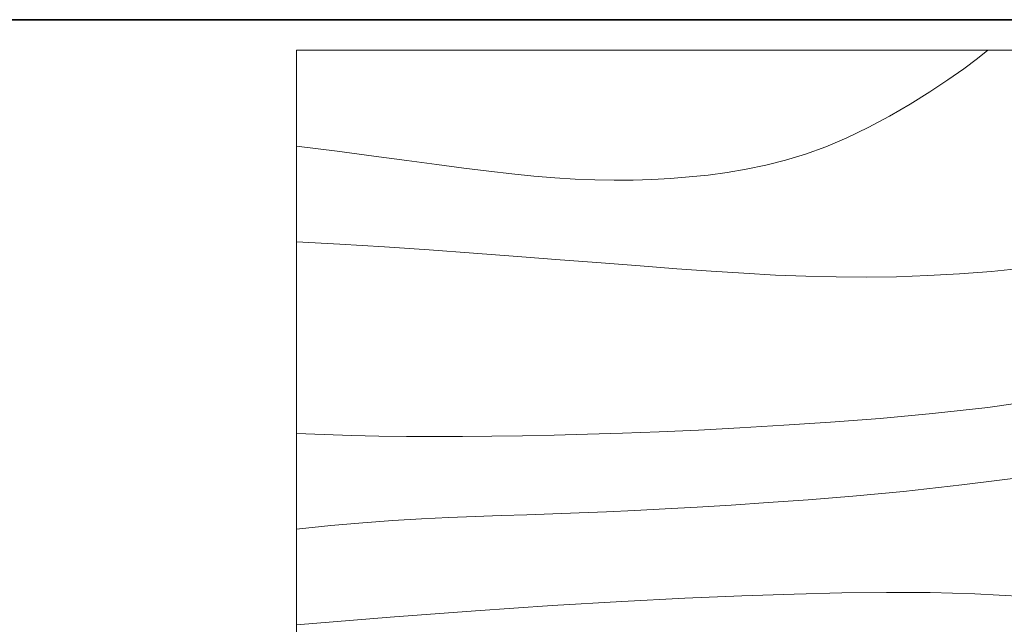
# Model space of a CAD drawing. Units: inches. Extents: x -128 to 854, y -395 to 398.
# Tile 40 of 61: x 270 to 296, y 170 to 187. Entities that reach past the tile are written whole.
import ezdxf

# ---------------------------------------------------------------- set-up
doc = ezdxf.new("R2010")
doc.units = ezdxf.units.IN
doc.header["$MEASUREMENT"] = 0
for name, color, linetype, lineweight in [('A-ANNO-DIMS', 2, 'Continuous', 18), ('A-FURN', 8, 'Continuous', 18), ('A-WALL', 4, 'Continuous', 35)]:
    doc.layers.add(name, color=color, linetype=linetype, lineweight=lineweight)
doc.styles.get("Standard").update_dxf_attribs({"font": 'arial.ttf'})
doc.dimstyles.get("Standard").update_dxf_attribs({"dimtxt": 0.18, "dimasz": 0.18, "dimexe": 0.18, "dimexo": 0.0625, "dimgap": 0.09, "dimtad": 0, "dimtih": 1, "dimtoh": 1, "dimdec": 1, "dimzin": 0, "dimdsep": 46, "dimlunit": 4, "dimtxsty": 'Standard', "dimcen": 0.09, "dimclrd": 1, "dimclre": 2, "dimclrt": 6, "dimadec": 0, "dimazin": 0, "dimtfac": 1, "dimtdec": 1, "dimtofl": 0, "dimtmove": 0, "dimatfit": 3, "dimfxl": 1, "dimtfill": 2, "dimtfillclr": 3, "dimtolj": 1, "dimtzin": 0, "dimarcsym": 0})

# ---------------------------------------------------------------- blocks, each defined once
blk = doc.blocks.new('Table - Square Woodgrain 42 x 42 in.')
for points in [[(0, -4), (1.704, -4.2172), (3.2358, -4.4188), (4.615, -4.604), (5.8615, -4.7721), (6.9951, -4.9224), (8.0357, -5.0541), (9.0031, -5.1667), (9.9171, -5.2594), (10.7951, -5.3316), (11.6445, -5.3836), (12.4702, -5.4157), (13.277, -5.4283), (14.0698, -5.4217), (14.8535, -5.3964), (15.6331, -5.3526), (16.4133, -5.2908), (17.1986, -5.2103), (17.9913, -5.1062), (18.793, -4.9727), (19.6056, -4.8038), (20.4307, -4.5937), (21.2701, -4.3365), (22.1256, -4.0262), (22.9989, -3.6571), (23.888, -3.2272), (24.7756, -2.7516), (25.6408, -2.2491), (26.4624, -1.7387), (27.2195, -1.2395), (27.891, -0.7703), (28.456, -0.3501), (28.8934, 0.002)], [(0, -42), (0, 0), (42, 0), (42, -42)], [(0, -8), (1.8203, -8.1001), (3.6741, -8.2149), (5.5411, -8.3408), (7.4011, -8.4741), (9.2339, -8.6112), (11.0193, -8.7484), (12.7371, -8.8821), (14.3671, -9.0086), (15.8954, -9.1246), (17.3337, -9.2278), (18.6997, -9.3159), (20.0116, -9.387), (21.2871, -9.4389), (22.5442, -9.4696), (23.8008, -9.477), (25.0749, -9.459), (26.3791, -9.4137), (27.7049, -9.3403), (29.0383, -9.2382), (30.3655, -9.1068)], [(31.3004, -14.5731), (28.8832, -14.9161), (26.577, -15.1775), (24.3858, -15.3768), (22.3136, -15.5332), (20.3622, -15.6632), (18.5254, -15.7718), (16.7947, -15.8612), (15.1618, -15.9338), (13.6183, -15.9916), (12.1558, -16.0369), (10.7659, -16.0718), (9.4403, -16.0987), (8.1703, -16.1191), (6.9461, -16.1325), (5.7577, -16.1377), (4.595, -16.1335), (3.4479, -16.1188), (2.3064, -16.0924), (1.1604, -16.0532), (0, -16)], [(30.6179, -17.7961), (27.8015, -18.1561), (25.3668, -18.4275), (23.2497, -18.6288), (21.3859, -18.7785), (19.7111, -18.8949), (18.1693, -18.9939), (16.7375, -19.0795), (15.401, -19.1534), (14.1449, -19.217), (12.9544, -19.2717), (11.8148, -19.3191), (10.7113, -19.3606), (9.6291, -19.3976), (8.5534, -19.4323), (7.47, -19.4689), (6.3643, -19.5122), (5.222, -19.5672), (4.0288, -19.6386), (2.7703, -19.7313), (1.4321, -19.8501), (0, -20)], [(0, -24), (3.9243, -23.6805), (7.4766, -23.4138), (10.6891, -23.1954), (13.5943, -23.0205), (16.2247, -22.8847), (18.6125, -22.7832), (20.7903, -22.7116), (22.7903, -22.6651), (24.6563, -22.642), (26.4764, -22.6507), (28.35, -22.7024), (30.3766, -22.8084), (32.6555, -22.98), (35.2861, -23.2283), (38.3678, -23.5645), (42, -24)]]:
    blk.add_lwpolyline(points)
blk = doc.blocks.new('*D55')
at = {"layer": 'A-ANNO-DIMS', "color": 0, "lineweight": -2, "transparency": 16777216}
for p, q in [((304.81, 186.741), (221.092, 186.741)), ((221.272, 181.741), (221.272, 131.873)), ((221.272, 77.741), (221.272, 127.608)), ((304.81, 72.741), (221.092, 72.741))]:
    blk.add_line(p, q, dxfattribs=at)
at = {"layer": 'A-ANNO-DIMS', "color": 0, "transparency": 16777216}
for points in [[(220.439, 181.741), (222.105, 181.741), (221.272, 186.741)], [(220.439, 77.741), (222.105, 77.741), (221.272, 72.741)]]:
    blk.add_solid(points, dxfattribs=at)
at = {"layer": 'Defpoints', "color": 0, "transparency": 16777216}
for p in [(221.272, 186.741), (304.873, 186.741), (304.873, 72.741)]:
    blk.add_point(p, dxfattribs=at)
at = {"layer": 'A-ANNO-DIMS', "color": 0, "transparency": 16777216, "insert": (221.272, 129.741), "char_height": 4, "attachment_point": 5, "bg_fill": 1, "box_fill_scale": 1.25, "bg_fill_color": 3, "bg_fill_transparency": 0}
blk.add_mtext('\\A1;9\'-6"', dxfattribs=at)

msp = doc.modelspace()

# ---------------------------------------------------------------- linework, layer by layer
at = {"layer": 'A-WALL'}
msp.add_line((304.873, 186.741), (220.42, 186.741), dxfattribs=at)

# ---------------------------------------------------------------- block references
at = {"layer": 'A-FURN', "xscale": 0.6449685946951323, "yscale": 0.6449685946951323, "zscale": 0.6449685946951323}
msp.add_blockref('Table - Square Woodgrain 42 x 42 in.', (277.284, 185.917), dxfattribs=at)

# ---------------------------------------------------------------- dimensions: what is measured, and where the dimension line sits
at = {"layer": 'A-ANNO-DIMS'}
dim = msp.add_linear_dim(base=(221.272, 186.741), p1=(304.873, 72.741), p2=(304.873, 186.741), angle=90, dimstyle='Standard', override={"dimtxt": 4, "dimasz": 5, "dimclrd": 0, "dimclre": 0, "dimclrt": 0}, dxfattribs=at)
dim.commit()
dim.dimension.update_dxf_attribs({"geometry": '*D55', "text_midpoint": (221.272, 129.741)})

doc.saveas('drawing.dxf')
